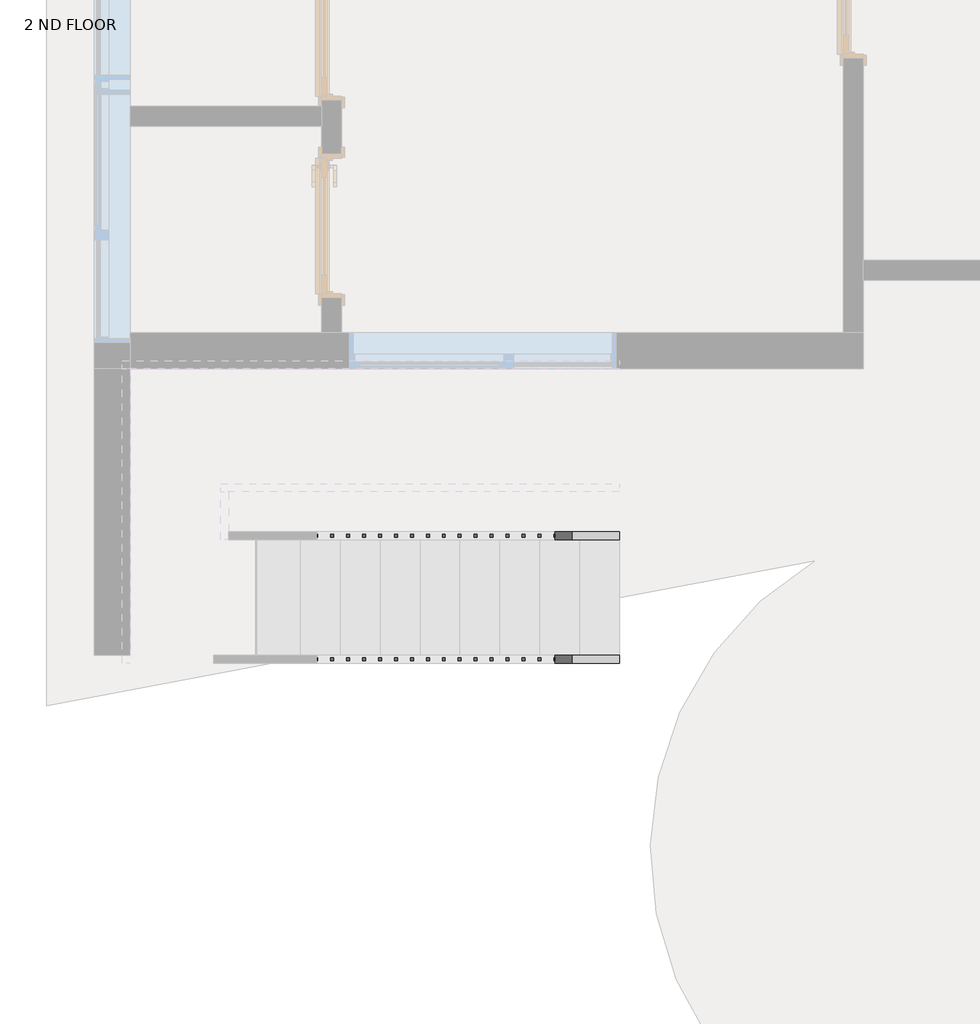
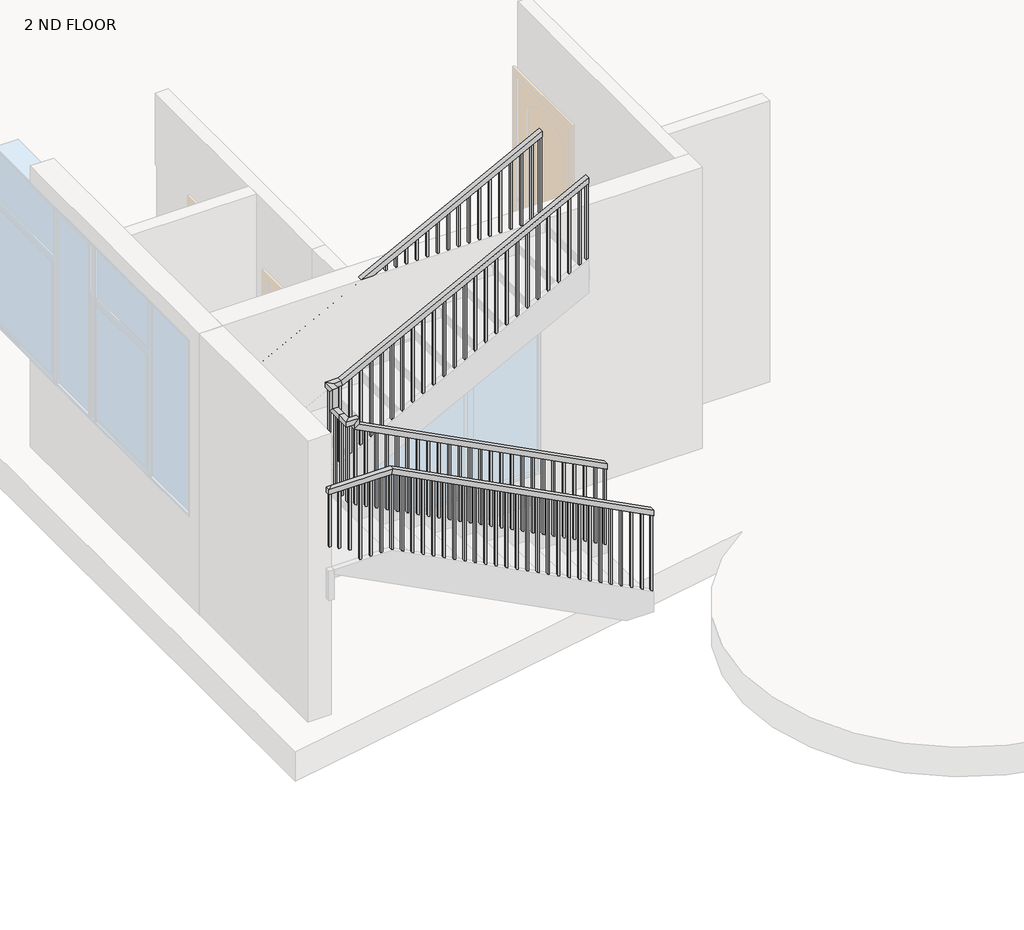
# One storey, part 3 of 4: 2 railings.
"""IFC4 building model written with IfcOpenShell, lengths in millimetres."""

from ifc_helpers import new_model, si_unit, frame, origin, place, context, project, spatial, polyline, outline, extrude, faceted_brep, element, save

model = new_model("IFC4")

# Units and contexts
model_context = context("Model", 3, world=origin())
ifc_project = project(units=[si_unit("LENGTHUNIT", "METRE", prefix="MILLI")], contexts=[model_context])

# Site, building, storey
site = spatial("IfcSite", under=ifc_project)
building = spatial("IfcBuilding", under=site)
storey = spatial("IfcBuildingStorey", under=building, Name="2 ND FLOOR", Elevation=6400.8)

# Railings
placement = place(None, origin())
element("IfcRailing", 1, ObjectType="Handrail - Rectangular", at=placement, inside=storey, context=model_context, shape_type="SolidModel", body=[
    faceted_brep([(-3117.2664982, -6914.3822004, 7446.8181818), (-3117.2664982, -6914.3822004, 7389.603028), (-3117.2664982, -6863.5822004, 7389.603028), (-3117.2664982, -6863.5822004, 7446.8181818), (-5530.2664982, -6914.3822004, 8697.1909091), (-5581.0664982, -6914.3822004, 8666.2993916), (-5581.0664982, -6863.5822004, 8666.2993916), (-5530.2664982, -6863.5822004, 8697.1909091), (-5657.2664982, -6787.3822004, 8712.2), (-5657.2664982, -6787.3822004, 8763.0), (-5657.2664982, -6685.7822004, 8763.0), (-5657.2664982, -6634.9822004, 8712.2), (-5606.4664982, -6787.3822004, 8712.2), (-5606.4664982, -6634.9822004, 8712.2), (-5606.4664982, -6787.3822004, 8763.0), (-5606.4664982, -6685.7822004, 8763.0), (-3117.2664982, -6558.7822004, 10210.8), (-3117.2664982, -6609.5822004, 10210.8), (-3117.2664982, -6609.5822004, 10153.5848461), (-3117.2664982, -6558.7822004, 10153.5848461), (-5517.8863767, -6558.7822004, 8909.6272727), (-5530.2664982, -6558.7822004, 8960.4272727), (-5517.8863767, -6609.5822004, 8909.6272727), (-5530.2664982, -6609.5822004, 8960.4272727), (-5530.2664982, -6914.3822004, 8763.0), (-5581.0664982, -6914.3822004, 8712.2), (-5581.0664982, -6863.5822004, 8712.2), (-5530.2664982, -6863.5822004, 8763.0), (-5657.2664982, -6914.3822004, 8763.0), (-5657.2664982, -6914.3822004, 8712.2), (-5606.4664982, -6863.5822004, 8712.2), (-5606.4664982, -6863.5822004, 8763.0), (-5657.2664982, -6685.7822004, 8960.4272727), (-5657.2664982, -6634.9822004, 8909.6272727), (-5606.4664982, -6634.9822004, 8909.6272727), (-5606.4664982, -6685.7822004, 8960.4272727), (-5657.2664982, -6558.7822004, 8960.4272727), (-5657.2664982, -6558.7822004, 8909.6272727), (-5606.4664982, -6609.5822004, 8909.6272727), (-5606.4664982, -6609.5822004, 8960.4272727)], [[[0, 1, 2, 3]], [[1, 0, 4, 5]], [[2, 1, 5, 6]], [[3, 2, 6, 7]], [[0, 3, 7, 4]], [[8, 9, 10, 11]], [[12, 8, 11, 13]], [[14, 12, 13, 15]], [[9, 14, 15, 10]], [[16, 17, 18, 19]], [[20, 21, 16, 19]], [[22, 20, 19, 18]], [[23, 22, 18, 17]], [[21, 23, 17, 16]], [[5, 4, 24, 25]], [[6, 5, 25, 26]], [[7, 6, 26, 27]], [[4, 7, 27, 24]], [[25, 24, 28, 29]], [[26, 25, 29, 30]], [[27, 26, 30, 31]], [[24, 27, 31, 28]], [[29, 28, 9, 8]], [[30, 29, 8, 12]], [[31, 30, 12, 14]], [[28, 31, 14, 9]], [[11, 10, 32, 33]], [[13, 11, 33, 34]], [[15, 13, 34, 35]], [[10, 15, 35, 32]], [[33, 32, 36, 37]], [[34, 33, 37, 38]], [[35, 34, 38, 39]], [[32, 35, 39, 36]], [[37, 36, 21, 20]], [[38, 37, 20, 22]], [[39, 38, 22, 23]], [[36, 39, 23, 21]]]),
    extrude(outline(polyline([(10119.0350734, -3183.9414982), (10109.1637098, -3202.9914982), (9324.8803899, -3202.9914982), (9334.7517536, -3183.9414982), (10119.0350734, -3183.9414982)])), frame((0.0, -6593.7072004, 0.0), z_axis=(0.0, 1.0, 0.0), x_axis=(0.0, 0.0, 1.0)), (0.0, 0.0, 1.0), 19.05),
    extrude(outline(polyline([(10066.3878007, -3285.5414982), (10056.516437, -3304.5914982), (9272.2331172, -3304.5914982), (9282.1044808, -3285.5414982), (10066.3878007, -3285.5414982)])), frame((0.0, -6593.7072004, 0.0), z_axis=(0.0, 1.0, 0.0), x_axis=(0.0, 0.0, 1.0)), (0.0, 0.0, 1.0), 19.05),
    extrude(outline(polyline([(10013.740528, -3387.1414982), (10003.8691643, -3406.1914982), (9219.5858445, -3406.1914982), (9229.4572081, -3387.1414982), (10013.740528, -3387.1414982)])), frame((0.0, -6593.7072004, 0.0), z_axis=(0.0, 1.0, 0.0), x_axis=(0.0, 0.0, 1.0)), (0.0, 0.0, 1.0), 19.05),
    extrude(outline(polyline([(9961.0932552, -3488.7414982), (9951.2218916, -3507.7914982), (9166.9385718, -3507.7914982), (9176.8099354, -3488.7414982), (9961.0932552, -3488.7414982)])), frame((0.0, -6593.7072004, 0.0), z_axis=(0.0, 1.0, 0.0), x_axis=(0.0, 0.0, 1.0)), (0.0, 0.0, 1.0), 19.05),
    extrude(outline(polyline([(9908.4459825, -3590.3414982), (9898.5746189, -3609.3914982), (9114.291299, -3609.3914982), (9124.1626627, -3590.3414982), (9908.4459825, -3590.3414982)])), frame((0.0, -6593.7072004, 0.0), z_axis=(0.0, 1.0, 0.0), x_axis=(0.0, 0.0, 1.0)), (0.0, 0.0, 1.0), 19.05),
    extrude(outline(polyline([(9855.7987098, -3691.9414982), (9845.9273461, -3710.9914982), (9061.6440263, -3710.9914982), (9071.5153899, -3691.9414982), (9855.7987098, -3691.9414982)])), frame((0.0, -6593.7072004, 0.0), z_axis=(0.0, 1.0, 0.0), x_axis=(0.0, 0.0, 1.0)), (0.0, 0.0, 1.0), 19.05),
    extrude(outline(polyline([(9803.151437, -3793.5414982), (9793.2800734, -3812.5914982), (9008.9967536, -3812.5914982), (9018.8681172, -3793.5414982), (9803.151437, -3793.5414982)])), frame((0.0, -6593.7072004, 0.0), z_axis=(0.0, 1.0, 0.0), x_axis=(0.0, 0.0, 1.0)), (0.0, 0.0, 1.0), 19.05),
    extrude(outline(polyline([(9750.5041643, -3895.1414982), (9740.6328007, -3914.1914982), (8956.3494808, -3914.1914982), (8966.2208445, -3895.1414982), (9750.5041643, -3895.1414982)])), frame((0.0, -6593.7072004, 0.0), z_axis=(0.0, 1.0, 0.0), x_axis=(0.0, 0.0, 1.0)), (0.0, 0.0, 1.0), 19.05),
    extrude(outline(polyline([(9697.8568916, -3996.7414982), (9687.985528, -4015.7914982), (8903.7022081, -4015.7914982), (8913.5735718, -3996.7414982), (9697.8568916, -3996.7414982)])), frame((0.0, -6593.7072004, 0.0), z_axis=(0.0, 1.0, 0.0), x_axis=(0.0, 0.0, 1.0)), (0.0, 0.0, 1.0), 19.05),
    extrude(outline(polyline([(9645.2096189, -4098.3414982), (9635.3382552, -4117.3914982), (8851.0549354, -4117.3914982), (8860.926299, -4098.3414982), (9645.2096189, -4098.3414982)])), frame((0.0, -6593.7072004, 0.0), z_axis=(0.0, 1.0, 0.0), x_axis=(0.0, 0.0, 1.0)), (0.0, 0.0, 1.0), 19.05),
    extrude(outline(polyline([(9592.5623461, -4199.9414982), (9582.6909825, -4218.9914982), (8798.4076627, -4218.9914982), (8808.2790263, -4199.9414982), (9592.5623461, -4199.9414982)])), frame((0.0, -6593.7072004, 0.0), z_axis=(0.0, 1.0, 0.0), x_axis=(0.0, 0.0, 1.0)), (0.0, 0.0, 1.0), 19.05),
    extrude(outline(polyline([(9539.9150734, -4301.5414982), (9530.0437098, -4320.5914982), (8745.7603899, -4320.5914982), (8755.6317536, -4301.5414982), (9539.9150734, -4301.5414982)])), frame((0.0, -6593.7072004, 0.0), z_axis=(0.0, 1.0, 0.0), x_axis=(0.0, 0.0, 1.0)), (0.0, 0.0, 1.0), 19.05),
    extrude(outline(polyline([(9487.2678007, -4403.1414982), (9477.396437, -4422.1914982), (8693.1131172, -4422.1914982), (8702.9844808, -4403.1414982), (9487.2678007, -4403.1414982)])), frame((0.0, -6593.7072004, 0.0), z_axis=(0.0, 1.0, 0.0), x_axis=(0.0, 0.0, 1.0)), (0.0, 0.0, 1.0), 19.05),
    extrude(outline(polyline([(9434.620528, -4504.7414982), (9424.7491643, -4523.7914982), (8640.4658445, -4523.7914982), (8650.3372081, -4504.7414982), (9434.620528, -4504.7414982)])), frame((0.0, -6593.7072004, 0.0), z_axis=(0.0, 1.0, 0.0), x_axis=(0.0, 0.0, 1.0)), (0.0, 0.0, 1.0), 19.05),
    extrude(outline(polyline([(9381.9732552, -4606.3414982), (9372.1018916, -4625.3914982), (8587.8185718, -4625.3914982), (8597.6899354, -4606.3414982), (9381.9732552, -4606.3414982)])), frame((0.0, -6593.7072004, 0.0), z_axis=(0.0, 1.0, 0.0), x_axis=(0.0, 0.0, 1.0)), (0.0, 0.0, 1.0), 19.05),
    extrude(outline(polyline([(9329.3259825, -4707.9414982), (9319.4546189, -4726.9914982), (8535.171299, -4726.9914982), (8545.0426627, -4707.9414982), (9329.3259825, -4707.9414982)])), frame((0.0, -6593.7072004, 0.0), z_axis=(0.0, 1.0, 0.0), x_axis=(0.0, 0.0, 1.0)), (0.0, 0.0, 1.0), 19.05),
    extrude(outline(polyline([(9276.6787098, -4809.5414982), (9266.8073461, -4828.5914982), (8482.5240263, -4828.5914982), (8492.3953899, -4809.5414982), (9276.6787098, -4809.5414982)])), frame((0.0, -6593.7072004, 0.0), z_axis=(0.0, 1.0, 0.0), x_axis=(0.0, 0.0, 1.0)), (0.0, 0.0, 1.0), 19.05),
    extrude(outline(polyline([(9224.031437, -4911.1414982), (9214.1600734, -4930.1914982), (8429.8767536, -4930.1914982), (8439.7481172, -4911.1414982), (9224.031437, -4911.1414982)])), frame((0.0, -6593.7072004, 0.0), z_axis=(0.0, 1.0, 0.0), x_axis=(0.0, 0.0, 1.0)), (0.0, 0.0, 1.0), 19.05),
    extrude(outline(polyline([(9171.3841643, -5012.7414982), (9161.5128007, -5031.7914982), (8377.2294808, -5031.7914982), (8387.1008445, -5012.7414982), (9171.3841643, -5012.7414982)])), frame((0.0, -6593.7072004, 0.0), z_axis=(0.0, 1.0, 0.0), x_axis=(0.0, 0.0, 1.0)), (0.0, 0.0, 1.0), 19.05),
    extrude(outline(polyline([(9118.7368916, -5114.3414982), (9108.865528, -5133.3914982), (8324.5822081, -5133.3914982), (8334.4535718, -5114.3414982), (9118.7368916, -5114.3414982)])), frame((0.0, -6593.7072004, 0.0), z_axis=(0.0, 1.0, 0.0), x_axis=(0.0, 0.0, 1.0)), (0.0, 0.0, 1.0), 19.05),
    extrude(outline(polyline([(9066.0896189, -5215.9414982), (9056.2182552, -5234.9914982), (8271.9349354, -5234.9914982), (8281.806299, -5215.9414982), (9066.0896189, -5215.9414982)])), frame((0.0, -6593.7072004, 0.0), z_axis=(0.0, 1.0, 0.0), x_axis=(0.0, 0.0, 1.0)), (0.0, 0.0, 1.0), 19.05),
    extrude(outline(polyline([(9013.4423461, -5317.5414982), (9003.5709825, -5336.5914982), (8219.2876627, -5336.5914982), (8229.1590263, -5317.5414982), (9013.4423461, -5317.5414982)])), frame((0.0, -6593.7072004, 0.0), z_axis=(0.0, 1.0, 0.0), x_axis=(0.0, 0.0, 1.0)), (0.0, 0.0, 1.0), 19.05),
    extrude(outline(polyline([(8960.7950734, -5419.1414982), (8950.9237098, -5438.1914982), (8166.6403899, -5438.1914982), (8176.5117536, -5419.1414982), (8960.7950734, -5419.1414982)])), frame((0.0, -6593.7072004, 0.0), z_axis=(0.0, 1.0, 0.0), x_axis=(0.0, 0.0, 1.0)), (0.0, 0.0, 1.0), 19.05),
    extrude(outline(polyline([(8908.1478007, -5520.7414982), (8898.276437, -5539.7914982), (8113.9931172, -5539.7914982), (8123.8644808, -5520.7414982), (8908.1478007, -5520.7414982)])), frame((0.0, -6593.7072004, 0.0), z_axis=(0.0, 1.0, 0.0), x_axis=(0.0, 0.0, 1.0)), (0.0, 0.0, 1.0), 19.05),
    extrude(outline(polyline([(-5622.3414982, -6695.3072004), (-5641.3914982, -6695.3072004), (-5641.3914982, -6676.2572004), (-5622.3414982, -6676.2572004), (-5622.3414982, -6695.3072004)])), frame((0.0, 0.0, 7924.8), z_axis=(0.0, 0.0, 1.0), x_axis=(1.0, 0.0, 0.0)), (0.0, 0.0, 1.0), 787.4),
    extrude(outline(polyline([(-5622.3414982, -6796.9072004), (-5641.3914982, -6796.9072004), (-5641.3914982, -6777.8572004), (-5622.3414982, -6777.8572004), (-5622.3414982, -6796.9072004)])), frame((0.0, 0.0, 7924.8), z_axis=(0.0, 0.0, 1.0), x_axis=(1.0, 0.0, 0.0)), (0.0, 0.0, 1.0), 787.4),
    extrude(outline(polyline([(8712.2, -5546.1414982), (8712.2, -5565.1914982), (7873.7899354, -5565.1914982), (7863.9185718, -5546.1414982), (8712.2, -5546.1414982)])), frame((0.0, -6898.5072004, 0.0), z_axis=(0.0, 1.0, 0.0), x_axis=(0.0, 0.0, 1.0)), (0.0, 0.0, 1.0), 19.05),
    extrude(outline(polyline([(8595.5546189, -5444.5414982), (8605.4259825, -5463.5914982), (7821.1426627, -5463.5914982), (7811.271299, -5444.5414982), (8595.5546189, -5444.5414982)])), frame((0.0, -6898.5072004, 0.0), z_axis=(0.0, 1.0, 0.0), x_axis=(0.0, 0.0, 1.0)), (0.0, 0.0, 1.0), 19.05),
    extrude(outline(polyline([(8542.9073461, -5342.9414982), (8552.7787098, -5361.9914982), (7768.4953899, -5361.9914982), (7758.6240263, -5342.9414982), (8542.9073461, -5342.9414982)])), frame((0.0, -6898.5072004, 0.0), z_axis=(0.0, 1.0, 0.0), x_axis=(0.0, 0.0, 1.0)), (0.0, 0.0, 1.0), 19.05),
    extrude(outline(polyline([(8490.2600734, -5241.3414982), (8500.131437, -5260.3914982), (7715.8481172, -5260.3914982), (7705.9767536, -5241.3414982), (8490.2600734, -5241.3414982)])), frame((0.0, -6898.5072004, 0.0), z_axis=(0.0, 1.0, 0.0), x_axis=(0.0, 0.0, 1.0)), (0.0, 0.0, 1.0), 19.05),
    extrude(outline(polyline([(8437.6128007, -5139.7414982), (8447.4841643, -5158.7914982), (7663.2008445, -5158.7914982), (7653.3294808, -5139.7414982), (8437.6128007, -5139.7414982)])), frame((0.0, -6898.5072004, 0.0), z_axis=(0.0, 1.0, 0.0), x_axis=(0.0, 0.0, 1.0)), (0.0, 0.0, 1.0), 19.05),
    extrude(outline(polyline([(8384.965528, -5038.1414982), (8394.8368916, -5057.1914982), (7610.5535718, -5057.1914982), (7600.6822081, -5038.1414982), (8384.965528, -5038.1414982)])), frame((0.0, -6898.5072004, 0.0), z_axis=(0.0, 1.0, 0.0), x_axis=(0.0, 0.0, 1.0)), (0.0, 0.0, 1.0), 19.05),
    extrude(outline(polyline([(8332.3182552, -4936.5414982), (8342.1896189, -4955.5914982), (7557.906299, -4955.5914982), (7548.0349354, -4936.5414982), (8332.3182552, -4936.5414982)])), frame((0.0, -6898.5072004, 0.0), z_axis=(0.0, 1.0, 0.0), x_axis=(0.0, 0.0, 1.0)), (0.0, 0.0, 1.0), 19.05),
    extrude(outline(polyline([(8279.6709825, -4834.9414982), (8289.5423461, -4853.9914982), (7505.2590263, -4853.9914982), (7495.3876627, -4834.9414982), (8279.6709825, -4834.9414982)])), frame((0.0, -6898.5072004, 0.0), z_axis=(0.0, 1.0, 0.0), x_axis=(0.0, 0.0, 1.0)), (0.0, 0.0, 1.0), 19.05),
    extrude(outline(polyline([(8227.0237098, -4733.3414982), (8236.8950734, -4752.3914982), (7452.6117536, -4752.3914982), (7442.7403899, -4733.3414982), (8227.0237098, -4733.3414982)])), frame((0.0, -6898.5072004, 0.0), z_axis=(0.0, 1.0, 0.0), x_axis=(0.0, 0.0, 1.0)), (0.0, 0.0, 1.0), 19.05),
    extrude(outline(polyline([(8174.376437, -4631.7414982), (8184.2478007, -4650.7914982), (7399.9644808, -4650.7914982), (7390.0931172, -4631.7414982), (8174.376437, -4631.7414982)])), frame((0.0, -6898.5072004, 0.0), z_axis=(0.0, 1.0, 0.0), x_axis=(0.0, 0.0, 1.0)), (0.0, 0.0, 1.0), 19.05),
    extrude(outline(polyline([(8121.7291643, -4530.1414982), (8131.600528, -4549.1914982), (7347.3172081, -4549.1914982), (7337.4458445, -4530.1414982), (8121.7291643, -4530.1414982)])), frame((0.0, -6898.5072004, 0.0), z_axis=(0.0, 1.0, 0.0), x_axis=(0.0, 0.0, 1.0)), (0.0, 0.0, 1.0), 19.05),
    extrude(outline(polyline([(8069.0818916, -4428.5414982), (8078.9532552, -4447.5914982), (7294.6699354, -4447.5914982), (7284.7985718, -4428.5414982), (8069.0818916, -4428.5414982)])), frame((0.0, -6898.5072004, 0.0), z_axis=(0.0, 1.0, 0.0), x_axis=(0.0, 0.0, 1.0)), (0.0, 0.0, 1.0), 19.05),
    extrude(outline(polyline([(8016.4346189, -4326.9414982), (8026.3059825, -4345.9914982), (7242.0226627, -4345.9914982), (7232.151299, -4326.9414982), (8016.4346189, -4326.9414982)])), frame((0.0, -6898.5072004, 0.0), z_axis=(0.0, 1.0, 0.0), x_axis=(0.0, 0.0, 1.0)), (0.0, 0.0, 1.0), 19.05),
    extrude(outline(polyline([(7963.7873461, -4225.3414982), (7973.6587098, -4244.3914982), (7189.3753899, -4244.3914982), (7179.5040263, -4225.3414982), (7963.7873461, -4225.3414982)])), frame((0.0, -6898.5072004, 0.0), z_axis=(0.0, 1.0, 0.0), x_axis=(0.0, 0.0, 1.0)), (0.0, 0.0, 1.0), 19.05),
    extrude(outline(polyline([(7911.1400734, -4123.7414982), (7921.011437, -4142.7914982), (7136.7281172, -4142.7914982), (7126.8567536, -4123.7414982), (7911.1400734, -4123.7414982)])), frame((0.0, -6898.5072004, 0.0), z_axis=(0.0, 1.0, 0.0), x_axis=(0.0, 0.0, 1.0)), (0.0, 0.0, 1.0), 19.05),
    extrude(outline(polyline([(7858.4928007, -4022.1414982), (7868.3641643, -4041.1914982), (7084.0808445, -4041.1914982), (7074.2094808, -4022.1414982), (7858.4928007, -4022.1414982)])), frame((0.0, -6898.5072004, 0.0), z_axis=(0.0, 1.0, 0.0), x_axis=(0.0, 0.0, 1.0)), (0.0, 0.0, 1.0), 19.05),
    extrude(outline(polyline([(7805.845528, -3920.5414982), (7815.7168916, -3939.5914982), (7031.4335718, -3939.5914982), (7021.5622081, -3920.5414982), (7805.845528, -3920.5414982)])), frame((0.0, -6898.5072004, 0.0), z_axis=(0.0, 1.0, 0.0), x_axis=(0.0, 0.0, 1.0)), (0.0, 0.0, 1.0), 19.05),
    extrude(outline(polyline([(7753.1982552, -3818.9414982), (7763.0696189, -3837.9914982), (6978.786299, -3837.9914982), (6968.9149354, -3818.9414982), (7753.1982552, -3818.9414982)])), frame((0.0, -6898.5072004, 0.0), z_axis=(0.0, 1.0, 0.0), x_axis=(0.0, 0.0, 1.0)), (0.0, 0.0, 1.0), 19.05),
    extrude(outline(polyline([(7700.5509825, -3717.3414982), (7710.4223461, -3736.3914982), (6926.1390263, -3736.3914982), (6916.2676627, -3717.3414982), (7700.5509825, -3717.3414982)])), frame((0.0, -6898.5072004, 0.0), z_axis=(0.0, 1.0, 0.0), x_axis=(0.0, 0.0, 1.0)), (0.0, 0.0, 1.0), 19.05),
    extrude(outline(polyline([(7647.9037098, -3615.7414982), (7657.7750734, -3634.7914982), (6873.4917536, -3634.7914982), (6863.6203899, -3615.7414982), (7647.9037098, -3615.7414982)])), frame((0.0, -6898.5072004, 0.0), z_axis=(0.0, 1.0, 0.0), x_axis=(0.0, 0.0, 1.0)), (0.0, 0.0, 1.0), 19.05),
    extrude(outline(polyline([(7595.256437, -3514.1414982), (7605.1278007, -3533.1914982), (6820.8444808, -3533.1914982), (6810.9731172, -3514.1414982), (7595.256437, -3514.1414982)])), frame((0.0, -6898.5072004, 0.0), z_axis=(0.0, 1.0, 0.0), x_axis=(0.0, 0.0, 1.0)), (0.0, 0.0, 1.0), 19.05),
    extrude(outline(polyline([(7542.6091643, -3412.5414982), (7552.480528, -3431.5914982), (6768.1972081, -3431.5914982), (6758.3258445, -3412.5414982), (7542.6091643, -3412.5414982)])), frame((0.0, -6898.5072004, 0.0), z_axis=(0.0, 1.0, 0.0), x_axis=(0.0, 0.0, 1.0)), (0.0, 0.0, 1.0), 19.05),
    extrude(outline(polyline([(7489.9618916, -3310.9414982), (7499.8332552, -3329.9914982), (6715.5499354, -3329.9914982), (6705.6785718, -3310.9414982), (7489.9618916, -3310.9414982)])), frame((0.0, -6898.5072004, 0.0), z_axis=(0.0, 1.0, 0.0), x_axis=(0.0, 0.0, 1.0)), (0.0, 0.0, 1.0), 19.05),
    extrude(outline(polyline([(7437.3146189, -3209.3414982), (7447.1859825, -3228.3914982), (6662.9026627, -3228.3914982), (6653.031299, -3209.3414982), (7437.3146189, -3209.3414982)])), frame((0.0, -6898.5072004, 0.0), z_axis=(0.0, 1.0, 0.0), x_axis=(0.0, 0.0, 1.0)), (0.0, 0.0, 1.0), 19.05),
    extrude(outline(polyline([(-6593.7072004, 8909.6272727), (-6574.6572004, 8909.6272727), (-6574.6572004, 8071.2172081), (-6593.7072004, 8061.3458445), (-6593.7072004, 8909.6272727)])), frame((-5641.3914982, 0.0, 0.0), z_axis=(1.0, 0.0, 0.0), x_axis=(0.0, 1.0, 0.0)), (0.0, 0.0, 1.0), 19.05),
    extrude(outline(polyline([(-5622.3414982, -6879.4572004), (-5622.3414982, -6898.5072004), (-5641.3914982, -6898.5072004), (-5641.3914982, -6879.4572004), (-5622.3414982, -6879.4572004)])), frame((0.0, 0.0, 7924.8), z_axis=(0.0, 0.0, 1.0), x_axis=(1.0, 0.0, 0.0)), (0.0, 0.0, 1.0), 787.4),
    extrude(outline(polyline([(10153.5848461, -3117.2664982), (10143.7134825, -3136.3164982), (9359.4301627, -3136.3164982), (9369.3015263, -3117.2664982), (10153.5848461, -3117.2664982)])), frame((0.0, -6593.7072004, 0.0), z_axis=(0.0, 1.0, 0.0), x_axis=(0.0, 0.0, 1.0)), (0.0, 0.0, 1.0), 19.05),
    extrude(outline(polyline([(7389.603028, -3117.2664982), (7399.4743916, -3136.3164982), (6615.1910718, -3136.3164982), (6605.3197081, -3117.2664982), (7389.603028, -3117.2664982)])), frame((0.0, -6898.5072004, 0.0), z_axis=(0.0, 1.0, 0.0), x_axis=(0.0, 0.0, 1.0)), (0.0, 0.0, 1.0), 19.05),
])
element("IfcRailing", 2, ObjectType="Handrail - Rectangular", at=placement, inside=storey, context=model_context, shape_type="SolidModel", body=[
    faceted_brep([(-3117.2664982, -7701.7822004, 7446.8181818), (-3117.2664982, -7701.7822004, 7389.603028), (-3117.2664982, -7650.9822004, 7389.603028), (-3117.2664982, -7650.9822004, 7446.8181818), (-5657.2664982, -7701.7822004, 8763.0), (-5669.6466197, -7701.7822004, 8712.2), (-5669.6466197, -7650.9822004, 8712.2), (-5657.2664982, -7650.9822004, 8763.0), (-6283.3131972, -7701.7822004, 8712.2), (-6283.3131972, -7701.7822004, 8763.0), (-6283.3131972, -5773.9082131, 8763.0), (-6283.3131972, -5773.9082131, 8712.2), (-6232.5131972, -7650.9822004, 8712.2), (-6232.5131972, -5824.7082131, 8712.2), (-6232.5131972, -7650.9822004, 8763.0), (-6232.5131972, -5824.7082131, 8763.0), (-5911.2664982, -5773.9082131, 8763.0), (-5898.8863767, -5773.9082131, 8712.2), (-5898.8863767, -5824.7082131, 8712.2), (-5911.2664982, -5824.7082131, 8763.0), (-3117.2664982, -5773.9082131, 10210.8), (-3117.2664982, -5824.7082131, 10210.8), (-3117.2664982, -5824.7082131, 10153.5848461), (-3117.2664982, -5773.9082131, 10153.5848461)], [[[0, 1, 2, 3]], [[1, 0, 4, 5]], [[2, 1, 5, 6]], [[3, 2, 6, 7]], [[0, 3, 7, 4]], [[8, 9, 10, 11]], [[12, 8, 11, 13]], [[14, 12, 13, 15]], [[9, 14, 15, 10]], [[11, 10, 16, 17]], [[13, 11, 17, 18]], [[15, 13, 18, 19]], [[10, 15, 19, 16]], [[5, 4, 9, 8]], [[6, 5, 8, 12]], [[7, 6, 12, 14]], [[4, 7, 14, 9]], [[20, 21, 22, 23]], [[17, 16, 20, 23]], [[18, 17, 23, 22]], [[19, 18, 22, 21]], [[16, 19, 21, 20]]]),
    extrude(outline(polyline([(10100.6413294, -3219.4381972), (9316.3580095, -3219.4381972), (9326.2293732, -3200.3881972), (10110.512693, -3200.3881972), (10100.6413294, -3219.4381972)])), frame((0.0, -5808.8332131, 0.0), z_axis=(0.0, 1.0, 0.0), x_axis=(0.0, 0.0, 1.0)), (0.0, 0.0, 1.0), 19.05),
    extrude(outline(polyline([(10047.9940566, -3321.0381972), (9263.7107368, -3321.0381972), (9273.5821004, -3301.9881972), (10057.8654203, -3301.9881972), (10047.9940566, -3321.0381972)])), frame((0.0, -5808.8332131, 0.0), z_axis=(0.0, 1.0, 0.0), x_axis=(0.0, 0.0, 1.0)), (0.0, 0.0, 1.0), 19.05),
    extrude(outline(polyline([(9995.3467839, -3422.6381972), (9211.0634641, -3422.6381972), (9220.9348277, -3403.5881972), (10005.2181476, -3403.5881972), (9995.3467839, -3422.6381972)])), frame((0.0, -5808.8332131, 0.0), z_axis=(0.0, 1.0, 0.0), x_axis=(0.0, 0.0, 1.0)), (0.0, 0.0, 1.0), 19.05),
    extrude(outline(polyline([(9942.6995112, -3524.2381972), (9158.4161913, -3524.2381972), (9168.287555, -3505.1881972), (9952.5708748, -3505.1881972), (9942.6995112, -3524.2381972)])), frame((0.0, -5808.8332131, 0.0), z_axis=(0.0, 1.0, 0.0), x_axis=(0.0, 0.0, 1.0)), (0.0, 0.0, 1.0), 19.05),
    extrude(outline(polyline([(9890.0522385, -3625.8381972), (9105.7689186, -3625.8381972), (9115.6402823, -3606.7881972), (9899.9236021, -3606.7881972), (9890.0522385, -3625.8381972)])), frame((0.0, -5808.8332131, 0.0), z_axis=(0.0, 1.0, 0.0), x_axis=(0.0, 0.0, 1.0)), (0.0, 0.0, 1.0), 19.05),
    extrude(outline(polyline([(9837.4049657, -3727.4381972), (9053.1216459, -3727.4381972), (9062.9930095, -3708.3881972), (9847.2763294, -3708.3881972), (9837.4049657, -3727.4381972)])), frame((0.0, -5808.8332131, 0.0), z_axis=(0.0, 1.0, 0.0), x_axis=(0.0, 0.0, 1.0)), (0.0, 0.0, 1.0), 19.05),
    extrude(outline(polyline([(9784.757693, -3829.0381972), (9000.4743732, -3829.0381972), (9010.3457368, -3809.9881972), (9794.6290566, -3809.9881972), (9784.757693, -3829.0381972)])), frame((0.0, -5808.8332131, 0.0), z_axis=(0.0, 1.0, 0.0), x_axis=(0.0, 0.0, 1.0)), (0.0, 0.0, 1.0), 19.05),
    extrude(outline(polyline([(9732.1104203, -3930.6381972), (8947.8271004, -3930.6381972), (8957.6984641, -3911.5881972), (9741.9817839, -3911.5881972), (9732.1104203, -3930.6381972)])), frame((0.0, -5808.8332131, 0.0), z_axis=(0.0, 1.0, 0.0), x_axis=(0.0, 0.0, 1.0)), (0.0, 0.0, 1.0), 19.05),
    extrude(outline(polyline([(9679.4631476, -4032.2381972), (8895.1798277, -4032.2381972), (8905.0511913, -4013.1881972), (9689.3345112, -4013.1881972), (9679.4631476, -4032.2381972)])), frame((0.0, -5808.8332131, 0.0), z_axis=(0.0, 1.0, 0.0), x_axis=(0.0, 0.0, 1.0)), (0.0, 0.0, 1.0), 19.05),
    extrude(outline(polyline([(9626.8158748, -4133.8381972), (8842.532555, -4133.8381972), (8852.4039186, -4114.7881972), (9636.6872385, -4114.7881972), (9626.8158748, -4133.8381972)])), frame((0.0, -5808.8332131, 0.0), z_axis=(0.0, 1.0, 0.0), x_axis=(0.0, 0.0, 1.0)), (0.0, 0.0, 1.0), 19.05),
    extrude(outline(polyline([(9574.1686021, -4235.4381972), (8789.8852823, -4235.4381972), (8799.7566459, -4216.3881972), (9584.0399657, -4216.3881972), (9574.1686021, -4235.4381972)])), frame((0.0, -5808.8332131, 0.0), z_axis=(0.0, 1.0, 0.0), x_axis=(0.0, 0.0, 1.0)), (0.0, 0.0, 1.0), 19.05),
    extrude(outline(polyline([(9521.5213294, -4337.0381972), (8737.2380095, -4337.0381972), (8747.1093732, -4317.9881972), (9531.392693, -4317.9881972), (9521.5213294, -4337.0381972)])), frame((0.0, -5808.8332131, 0.0), z_axis=(0.0, 1.0, 0.0), x_axis=(0.0, 0.0, 1.0)), (0.0, 0.0, 1.0), 19.05),
    extrude(outline(polyline([(9468.8740566, -4438.6381972), (8684.5907368, -4438.6381972), (8694.4621004, -4419.5881972), (9478.7454203, -4419.5881972), (9468.8740566, -4438.6381972)])), frame((0.0, -5808.8332131, 0.0), z_axis=(0.0, 1.0, 0.0), x_axis=(0.0, 0.0, 1.0)), (0.0, 0.0, 1.0), 19.05),
    extrude(outline(polyline([(9416.2267839, -4540.2381972), (8631.9434641, -4540.2381972), (8641.8148277, -4521.1881972), (9426.0981476, -4521.1881972), (9416.2267839, -4540.2381972)])), frame((0.0, -5808.8332131, 0.0), z_axis=(0.0, 1.0, 0.0), x_axis=(0.0, 0.0, 1.0)), (0.0, 0.0, 1.0), 19.05),
    extrude(outline(polyline([(9363.5795112, -4641.8381972), (8579.2961913, -4641.8381972), (8589.167555, -4622.7881972), (9373.4508748, -4622.7881972), (9363.5795112, -4641.8381972)])), frame((0.0, -5808.8332131, 0.0), z_axis=(0.0, 1.0, 0.0), x_axis=(0.0, 0.0, 1.0)), (0.0, 0.0, 1.0), 19.05),
    extrude(outline(polyline([(9310.9322385, -4743.4381972), (8526.6489186, -4743.4381972), (8536.5202823, -4724.3881972), (9320.8036021, -4724.3881972), (9310.9322385, -4743.4381972)])), frame((0.0, -5808.8332131, 0.0), z_axis=(0.0, 1.0, 0.0), x_axis=(0.0, 0.0, 1.0)), (0.0, 0.0, 1.0), 19.05),
    extrude(outline(polyline([(9258.2849657, -4845.0381972), (8474.0016459, -4845.0381972), (8483.8730095, -4825.9881972), (9268.1563294, -4825.9881972), (9258.2849657, -4845.0381972)])), frame((0.0, -5808.8332131, 0.0), z_axis=(0.0, 1.0, 0.0), x_axis=(0.0, 0.0, 1.0)), (0.0, 0.0, 1.0), 19.05),
    extrude(outline(polyline([(9205.637693, -4946.6381972), (8421.3543732, -4946.6381972), (8431.2257368, -4927.5881972), (9215.5090566, -4927.5881972), (9205.637693, -4946.6381972)])), frame((0.0, -5808.8332131, 0.0), z_axis=(0.0, 1.0, 0.0), x_axis=(0.0, 0.0, 1.0)), (0.0, 0.0, 1.0), 19.05),
    extrude(outline(polyline([(9152.9904203, -5048.2381972), (8368.7071004, -5048.2381972), (8378.5784641, -5029.1881972), (9162.8617839, -5029.1881972), (9152.9904203, -5048.2381972)])), frame((0.0, -5808.8332131, 0.0), z_axis=(0.0, 1.0, 0.0), x_axis=(0.0, 0.0, 1.0)), (0.0, 0.0, 1.0), 19.05),
    extrude(outline(polyline([(9100.3431476, -5149.8381972), (8316.0598277, -5149.8381972), (8325.9311913, -5130.7881972), (9110.2145112, -5130.7881972), (9100.3431476, -5149.8381972)])), frame((0.0, -5808.8332131, 0.0), z_axis=(0.0, 1.0, 0.0), x_axis=(0.0, 0.0, 1.0)), (0.0, 0.0, 1.0), 19.05),
    extrude(outline(polyline([(9047.6958748, -5251.4381972), (8263.412555, -5251.4381972), (8273.2839186, -5232.3881972), (9057.5672385, -5232.3881972), (9047.6958748, -5251.4381972)])), frame((0.0, -5808.8332131, 0.0), z_axis=(0.0, 1.0, 0.0), x_axis=(0.0, 0.0, 1.0)), (0.0, 0.0, 1.0), 19.05),
    extrude(outline(polyline([(8995.0486021, -5353.0381972), (8210.7652823, -5353.0381972), (8220.6366459, -5333.9881972), (9004.9199657, -5333.9881972), (8995.0486021, -5353.0381972)])), frame((0.0, -5808.8332131, 0.0), z_axis=(0.0, 1.0, 0.0), x_axis=(0.0, 0.0, 1.0)), (0.0, 0.0, 1.0), 19.05),
    extrude(outline(polyline([(8942.4013294, -5454.6381972), (8158.1180095, -5454.6381972), (8167.9893732, -5435.5881972), (8952.272693, -5435.5881972), (8942.4013294, -5454.6381972)])), frame((0.0, -5808.8332131, 0.0), z_axis=(0.0, 1.0, 0.0), x_axis=(0.0, 0.0, 1.0)), (0.0, 0.0, 1.0), 19.05),
    extrude(outline(polyline([(8889.7540566, -5556.2381972), (8105.4707368, -5556.2381972), (8115.3421004, -5537.1881972), (8899.6254203, -5537.1881972), (8889.7540566, -5556.2381972)])), frame((0.0, -5808.8332131, 0.0), z_axis=(0.0, 1.0, 0.0), x_axis=(0.0, 0.0, 1.0)), (0.0, 0.0, 1.0), 19.05),
    extrude(outline(polyline([(8837.1067839, -5657.8381972), (8052.8234641, -5657.8381972), (8062.6948277, -5638.7881972), (8846.9781476, -5638.7881972), (8837.1067839, -5657.8381972)])), frame((0.0, -5808.8332131, 0.0), z_axis=(0.0, 1.0, 0.0), x_axis=(0.0, 0.0, 1.0)), (0.0, 0.0, 1.0), 19.05),
    extrude(outline(polyline([(8784.4595112, -5759.4381972), (8000.1761913, -5759.4381972), (8010.047555, -5740.3881972), (8794.3308748, -5740.3881972), (8784.4595112, -5759.4381972)])), frame((0.0, -5808.8332131, 0.0), z_axis=(0.0, 1.0, 0.0), x_axis=(0.0, 0.0, 1.0)), (0.0, 0.0, 1.0), 19.05),
    extrude(outline(polyline([(8731.8122385, -5861.0381972), (7947.5289186, -5861.0381972), (7957.4002823, -5841.9881972), (8741.6836021, -5841.9881972), (8731.8122385, -5861.0381972)])), frame((0.0, -5808.8332131, 0.0), z_axis=(0.0, 1.0, 0.0), x_axis=(0.0, 0.0, 1.0)), (0.0, 0.0, 1.0), 19.05),
    extrude(outline(polyline([(8712.2, -5962.6381972), (7894.8816459, -5962.6381972), (7904.7530095, -5943.5881972), (8712.2, -5943.5881972), (8712.2, -5962.6381972)])), frame((0.0, -5808.8332131, 0.0), z_axis=(0.0, 1.0, 0.0), x_axis=(0.0, 0.0, 1.0)), (0.0, 0.0, 1.0), 19.05),
    extrude(outline(polyline([(8712.2, -6064.2381972), (7842.2343732, -6064.2381972), (7852.1057368, -6045.1881972), (8712.2, -6045.1881972), (8712.2, -6064.2381972)])), frame((0.0, -5808.8332131, 0.0), z_axis=(0.0, 1.0, 0.0), x_axis=(0.0, 0.0, 1.0)), (0.0, 0.0, 1.0), 19.05),
    extrude(outline(polyline([(8712.2, -6165.8381972), (7789.5871004, -6165.8381972), (7799.4584641, -6146.7881972), (8712.2, -6146.7881972), (8712.2, -6165.8381972)])), frame((0.0, -5808.8332131, 0.0), z_axis=(0.0, 1.0, 0.0), x_axis=(0.0, 0.0, 1.0)), (0.0, 0.0, 1.0), 19.05),
    extrude(outline(polyline([(-6267.4381972, -5857.1072004), (-6267.4381972, -5838.0572004), (-6248.3881972, -5838.0572004), (-6248.3881972, -5857.1072004), (-6267.4381972, -5857.1072004)])), frame((0.0, 0.0, 7924.8), z_axis=(0.0, 0.0, 1.0), x_axis=(1.0, 0.0, 0.0)), (0.0, 0.0, 1.0), 787.4),
    extrude(outline(polyline([(-6267.4381972, -5958.7072004), (-6267.4381972, -5939.6572004), (-6248.3881972, -5939.6572004), (-6248.3881972, -5958.7072004), (-6267.4381972, -5958.7072004)])), frame((0.0, 0.0, 7924.8), z_axis=(0.0, 0.0, 1.0), x_axis=(1.0, 0.0, 0.0)), (0.0, 0.0, 1.0), 787.4),
    extrude(outline(polyline([(-6267.4381972, -6060.3072004), (-6267.4381972, -6041.2572004), (-6248.3881972, -6041.2572004), (-6248.3881972, -6060.3072004), (-6267.4381972, -6060.3072004)])), frame((0.0, 0.0, 7924.8), z_axis=(0.0, 0.0, 1.0), x_axis=(1.0, 0.0, 0.0)), (0.0, 0.0, 1.0), 787.4),
    extrude(outline(polyline([(-6267.4381972, -6161.9072004), (-6267.4381972, -6142.8572004), (-6248.3881972, -6142.8572004), (-6248.3881972, -6161.9072004), (-6267.4381972, -6161.9072004)])), frame((0.0, 0.0, 7924.8), z_axis=(0.0, 0.0, 1.0), x_axis=(1.0, 0.0, 0.0)), (0.0, 0.0, 1.0), 787.4),
    extrude(outline(polyline([(-6267.4381972, -6263.5072004), (-6267.4381972, -6244.4572004), (-6248.3881972, -6244.4572004), (-6248.3881972, -6263.5072004), (-6267.4381972, -6263.5072004)])), frame((0.0, 0.0, 7924.8), z_axis=(0.0, 0.0, 1.0), x_axis=(1.0, 0.0, 0.0)), (0.0, 0.0, 1.0), 787.4),
    extrude(outline(polyline([(-6267.4381972, -6365.1072004), (-6267.4381972, -6346.0572004), (-6248.3881972, -6346.0572004), (-6248.3881972, -6365.1072004), (-6267.4381972, -6365.1072004)])), frame((0.0, 0.0, 7924.8), z_axis=(0.0, 0.0, 1.0), x_axis=(1.0, 0.0, 0.0)), (0.0, 0.0, 1.0), 787.4),
    extrude(outline(polyline([(-6267.4381972, -6466.7072004), (-6267.4381972, -6447.6572004), (-6248.3881972, -6447.6572004), (-6248.3881972, -6466.7072004), (-6267.4381972, -6466.7072004)])), frame((0.0, 0.0, 7924.8), z_axis=(0.0, 0.0, 1.0), x_axis=(1.0, 0.0, 0.0)), (0.0, 0.0, 1.0), 787.4),
    extrude(outline(polyline([(-6267.4381972, -6568.3072004), (-6267.4381972, -6549.2572004), (-6248.3881972, -6549.2572004), (-6248.3881972, -6568.3072004), (-6267.4381972, -6568.3072004)])), frame((0.0, 0.0, 7924.8), z_axis=(0.0, 0.0, 1.0), x_axis=(1.0, 0.0, 0.0)), (0.0, 0.0, 1.0), 787.4),
    extrude(outline(polyline([(-6267.4381972, -6669.9072004), (-6267.4381972, -6650.8572004), (-6248.3881972, -6650.8572004), (-6248.3881972, -6669.9072004), (-6267.4381972, -6669.9072004)])), frame((0.0, 0.0, 7924.8), z_axis=(0.0, 0.0, 1.0), x_axis=(1.0, 0.0, 0.0)), (0.0, 0.0, 1.0), 787.4),
    extrude(outline(polyline([(-6267.4381972, -6771.5072004), (-6267.4381972, -6752.4572004), (-6248.3881972, -6752.4572004), (-6248.3881972, -6771.5072004), (-6267.4381972, -6771.5072004)])), frame((0.0, 0.0, 7924.8), z_axis=(0.0, 0.0, 1.0), x_axis=(1.0, 0.0, 0.0)), (0.0, 0.0, 1.0), 787.4),
    extrude(outline(polyline([(-6267.4381972, -6873.1072004), (-6267.4381972, -6854.0572004), (-6248.3881972, -6854.0572004), (-6248.3881972, -6873.1072004), (-6267.4381972, -6873.1072004)])), frame((0.0, 0.0, 7924.8), z_axis=(0.0, 0.0, 1.0), x_axis=(1.0, 0.0, 0.0)), (0.0, 0.0, 1.0), 787.4),
    extrude(outline(polyline([(-6267.4381972, -6974.7072004), (-6267.4381972, -6955.6572004), (-6248.3881972, -6955.6572004), (-6248.3881972, -6974.7072004), (-6267.4381972, -6974.7072004)])), frame((0.0, 0.0, 7924.8), z_axis=(0.0, 0.0, 1.0), x_axis=(1.0, 0.0, 0.0)), (0.0, 0.0, 1.0), 787.4),
    extrude(outline(polyline([(-6267.4381972, -7076.3072004), (-6267.4381972, -7057.2572004), (-6248.3881972, -7057.2572004), (-6248.3881972, -7076.3072004), (-6267.4381972, -7076.3072004)])), frame((0.0, 0.0, 7924.8), z_axis=(0.0, 0.0, 1.0), x_axis=(1.0, 0.0, 0.0)), (0.0, 0.0, 1.0), 787.4),
    extrude(outline(polyline([(-6267.4381972, -7177.9072004), (-6267.4381972, -7158.8572004), (-6248.3881972, -7158.8572004), (-6248.3881972, -7177.9072004), (-6267.4381972, -7177.9072004)])), frame((0.0, 0.0, 7924.8), z_axis=(0.0, 0.0, 1.0), x_axis=(1.0, 0.0, 0.0)), (0.0, 0.0, 1.0), 787.4),
    extrude(outline(polyline([(-6267.4381972, -7279.5072004), (-6267.4381972, -7260.4572004), (-6248.3881972, -7260.4572004), (-6248.3881972, -7279.5072004), (-6267.4381972, -7279.5072004)])), frame((0.0, 0.0, 7924.8), z_axis=(0.0, 0.0, 1.0), x_axis=(1.0, 0.0, 0.0)), (0.0, 0.0, 1.0), 787.4),
    extrude(outline(polyline([(-6267.4381972, -7381.1072004), (-6267.4381972, -7362.0572004), (-6248.3881972, -7362.0572004), (-6248.3881972, -7381.1072004), (-6267.4381972, -7381.1072004)])), frame((0.0, 0.0, 7924.8), z_axis=(0.0, 0.0, 1.0), x_axis=(1.0, 0.0, 0.0)), (0.0, 0.0, 1.0), 787.4),
    extrude(outline(polyline([(-6267.4381972, -7482.7072004), (-6267.4381972, -7463.6572004), (-6248.3881972, -7463.6572004), (-6248.3881972, -7482.7072004), (-6267.4381972, -7482.7072004)])), frame((0.0, 0.0, 7924.8), z_axis=(0.0, 0.0, 1.0), x_axis=(1.0, 0.0, 0.0)), (0.0, 0.0, 1.0), 787.4),
    extrude(outline(polyline([(-6267.4381972, -7584.3072004), (-6267.4381972, -7565.2572004), (-6248.3881972, -7565.2572004), (-6248.3881972, -7584.3072004), (-6267.4381972, -7584.3072004)])), frame((0.0, 0.0, 7924.8), z_axis=(0.0, 0.0, 1.0), x_axis=(1.0, 0.0, 0.0)), (0.0, 0.0, 1.0), 787.4),
    extrude(outline(polyline([(-6155.7414982, -7685.9072004), (-6174.7914982, -7685.9072004), (-6174.7914982, -7666.8572004), (-6155.7414982, -7666.8572004), (-6155.7414982, -7685.9072004)])), frame((0.0, 0.0, 8111.8363636), z_axis=(0.0, 0.0, 1.0), x_axis=(1.0, 0.0, 0.0)), (0.0, 0.0, 1.0), 600.3636364),
    extrude(outline(polyline([(-6054.1414982, -7685.9072004), (-6073.1914982, -7685.9072004), (-6073.1914982, -7666.8572004), (-6054.1414982, -7666.8572004), (-6054.1414982, -7685.9072004)])), frame((0.0, 0.0, 8059.1890909), z_axis=(0.0, 0.0, 1.0), x_axis=(1.0, 0.0, 0.0)), (0.0, 0.0, 1.0), 653.0109091),
    extrude(outline(polyline([(-5952.5414982, -7685.9072004), (-5971.5914982, -7685.9072004), (-5971.5914982, -7666.8572004), (-5952.5414982, -7666.8572004), (-5952.5414982, -7685.9072004)])), frame((0.0, 0.0, 7924.8), z_axis=(0.0, 0.0, 1.0), x_axis=(1.0, 0.0, 0.0)), (0.0, 0.0, 1.0), 787.4),
    extrude(outline(polyline([(-5850.9414982, -7685.9072004), (-5869.9914982, -7685.9072004), (-5869.9914982, -7666.8572004), (-5850.9414982, -7666.8572004), (-5850.9414982, -7685.9072004)])), frame((0.0, 0.0, 7924.8), z_axis=(0.0, 0.0, 1.0), x_axis=(1.0, 0.0, 0.0)), (0.0, 0.0, 1.0), 787.4),
    extrude(outline(polyline([(-5749.3414982, -7685.9072004), (-5768.3914982, -7685.9072004), (-5768.3914982, -7666.8572004), (-5749.3414982, -7666.8572004), (-5749.3414982, -7685.9072004)])), frame((0.0, 0.0, 7924.8), z_axis=(0.0, 0.0, 1.0), x_axis=(1.0, 0.0, 0.0)), (0.0, 0.0, 1.0), 787.4),
    extrude(outline(polyline([(8710.720528, -5666.7914982), (7926.4372081, -5666.7914982), (7916.5658445, -5647.7414982), (8700.8491643, -5647.7414982), (8710.720528, -5666.7914982)])), frame((0.0, -7685.9072004, 0.0), z_axis=(0.0, 1.0, 0.0), x_axis=(0.0, 0.0, 1.0)), (0.0, 0.0, 1.0), 19.05),
    extrude(outline(polyline([(8658.0732552, -5565.1914982), (7873.7899354, -5565.1914982), (7863.9185718, -5546.1414982), (8648.2018916, -5546.1414982), (8658.0732552, -5565.1914982)])), frame((0.0, -7685.9072004, 0.0), z_axis=(0.0, 1.0, 0.0), x_axis=(0.0, 0.0, 1.0)), (0.0, 0.0, 1.0), 19.05),
    extrude(outline(polyline([(8605.4259825, -5463.5914982), (7821.1426627, -5463.5914982), (7811.271299, -5444.5414982), (8595.5546189, -5444.5414982), (8605.4259825, -5463.5914982)])), frame((0.0, -7685.9072004, 0.0), z_axis=(0.0, 1.0, 0.0), x_axis=(0.0, 0.0, 1.0)), (0.0, 0.0, 1.0), 19.05),
    extrude(outline(polyline([(8552.7787098, -5361.9914982), (7768.4953899, -5361.9914982), (7758.6240263, -5342.9414982), (8542.9073461, -5342.9414982), (8552.7787098, -5361.9914982)])), frame((0.0, -7685.9072004, 0.0), z_axis=(0.0, 1.0, 0.0), x_axis=(0.0, 0.0, 1.0)), (0.0, 0.0, 1.0), 19.05),
    extrude(outline(polyline([(8500.131437, -5260.3914982), (7715.8481172, -5260.3914982), (7705.9767536, -5241.3414982), (8490.2600734, -5241.3414982), (8500.131437, -5260.3914982)])), frame((0.0, -7685.9072004, 0.0), z_axis=(0.0, 1.0, 0.0), x_axis=(0.0, 0.0, 1.0)), (0.0, 0.0, 1.0), 19.05),
    extrude(outline(polyline([(8447.4841643, -5158.7914982), (7663.2008445, -5158.7914982), (7653.3294808, -5139.7414982), (8437.6128007, -5139.7414982), (8447.4841643, -5158.7914982)])), frame((0.0, -7685.9072004, 0.0), z_axis=(0.0, 1.0, 0.0), x_axis=(0.0, 0.0, 1.0)), (0.0, 0.0, 1.0), 19.05),
    extrude(outline(polyline([(8394.8368916, -5057.1914982), (7610.5535718, -5057.1914982), (7600.6822081, -5038.1414982), (8384.965528, -5038.1414982), (8394.8368916, -5057.1914982)])), frame((0.0, -7685.9072004, 0.0), z_axis=(0.0, 1.0, 0.0), x_axis=(0.0, 0.0, 1.0)), (0.0, 0.0, 1.0), 19.05),
    extrude(outline(polyline([(8342.1896189, -4955.5914982), (7557.906299, -4955.5914982), (7548.0349354, -4936.5414982), (8332.3182552, -4936.5414982), (8342.1896189, -4955.5914982)])), frame((0.0, -7685.9072004, 0.0), z_axis=(0.0, 1.0, 0.0), x_axis=(0.0, 0.0, 1.0)), (0.0, 0.0, 1.0), 19.05),
    extrude(outline(polyline([(8289.5423461, -4853.9914982), (7505.2590263, -4853.9914982), (7495.3876627, -4834.9414982), (8279.6709825, -4834.9414982), (8289.5423461, -4853.9914982)])), frame((0.0, -7685.9072004, 0.0), z_axis=(0.0, 1.0, 0.0), x_axis=(0.0, 0.0, 1.0)), (0.0, 0.0, 1.0), 19.05),
    extrude(outline(polyline([(8236.8950734, -4752.3914982), (7452.6117536, -4752.3914982), (7442.7403899, -4733.3414982), (8227.0237098, -4733.3414982), (8236.8950734, -4752.3914982)])), frame((0.0, -7685.9072004, 0.0), z_axis=(0.0, 1.0, 0.0), x_axis=(0.0, 0.0, 1.0)), (0.0, 0.0, 1.0), 19.05),
    extrude(outline(polyline([(8184.2478007, -4650.7914982), (7399.9644808, -4650.7914982), (7390.0931172, -4631.7414982), (8174.376437, -4631.7414982), (8184.2478007, -4650.7914982)])), frame((0.0, -7685.9072004, 0.0), z_axis=(0.0, 1.0, 0.0), x_axis=(0.0, 0.0, 1.0)), (0.0, 0.0, 1.0), 19.05),
    extrude(outline(polyline([(8131.600528, -4549.1914982), (7347.3172081, -4549.1914982), (7337.4458445, -4530.1414982), (8121.7291643, -4530.1414982), (8131.600528, -4549.1914982)])), frame((0.0, -7685.9072004, 0.0), z_axis=(0.0, 1.0, 0.0), x_axis=(0.0, 0.0, 1.0)), (0.0, 0.0, 1.0), 19.05),
    extrude(outline(polyline([(8078.9532552, -4447.5914982), (7294.6699354, -4447.5914982), (7284.7985718, -4428.5414982), (8069.0818916, -4428.5414982), (8078.9532552, -4447.5914982)])), frame((0.0, -7685.9072004, 0.0), z_axis=(0.0, 1.0, 0.0), x_axis=(0.0, 0.0, 1.0)), (0.0, 0.0, 1.0), 19.05),
    extrude(outline(polyline([(8026.3059825, -4345.9914982), (7242.0226627, -4345.9914982), (7232.151299, -4326.9414982), (8016.4346189, -4326.9414982), (8026.3059825, -4345.9914982)])), frame((0.0, -7685.9072004, 0.0), z_axis=(0.0, 1.0, 0.0), x_axis=(0.0, 0.0, 1.0)), (0.0, 0.0, 1.0), 19.05),
    extrude(outline(polyline([(7973.6587098, -4244.3914982), (7189.3753899, -4244.3914982), (7179.5040263, -4225.3414982), (7963.7873461, -4225.3414982), (7973.6587098, -4244.3914982)])), frame((0.0, -7685.9072004, 0.0), z_axis=(0.0, 1.0, 0.0), x_axis=(0.0, 0.0, 1.0)), (0.0, 0.0, 1.0), 19.05),
    extrude(outline(polyline([(7921.011437, -4142.7914982), (7136.7281172, -4142.7914982), (7126.8567536, -4123.7414982), (7911.1400734, -4123.7414982), (7921.011437, -4142.7914982)])), frame((0.0, -7685.9072004, 0.0), z_axis=(0.0, 1.0, 0.0), x_axis=(0.0, 0.0, 1.0)), (0.0, 0.0, 1.0), 19.05),
    extrude(outline(polyline([(7868.3641643, -4041.1914982), (7084.0808445, -4041.1914982), (7074.2094808, -4022.1414982), (7858.4928007, -4022.1414982), (7868.3641643, -4041.1914982)])), frame((0.0, -7685.9072004, 0.0), z_axis=(0.0, 1.0, 0.0), x_axis=(0.0, 0.0, 1.0)), (0.0, 0.0, 1.0), 19.05),
    extrude(outline(polyline([(7815.7168916, -3939.5914982), (7031.4335718, -3939.5914982), (7021.5622081, -3920.5414982), (7805.845528, -3920.5414982), (7815.7168916, -3939.5914982)])), frame((0.0, -7685.9072004, 0.0), z_axis=(0.0, 1.0, 0.0), x_axis=(0.0, 0.0, 1.0)), (0.0, 0.0, 1.0), 19.05),
    extrude(outline(polyline([(7763.0696189, -3837.9914982), (6978.786299, -3837.9914982), (6968.9149354, -3818.9414982), (7753.1982552, -3818.9414982), (7763.0696189, -3837.9914982)])), frame((0.0, -7685.9072004, 0.0), z_axis=(0.0, 1.0, 0.0), x_axis=(0.0, 0.0, 1.0)), (0.0, 0.0, 1.0), 19.05),
    extrude(outline(polyline([(7710.4223461, -3736.3914982), (6926.1390263, -3736.3914982), (6916.2676627, -3717.3414982), (7700.5509825, -3717.3414982), (7710.4223461, -3736.3914982)])), frame((0.0, -7685.9072004, 0.0), z_axis=(0.0, 1.0, 0.0), x_axis=(0.0, 0.0, 1.0)), (0.0, 0.0, 1.0), 19.05),
    extrude(outline(polyline([(7657.7750734, -3634.7914982), (6873.4917536, -3634.7914982), (6863.6203899, -3615.7414982), (7647.9037098, -3615.7414982), (7657.7750734, -3634.7914982)])), frame((0.0, -7685.9072004, 0.0), z_axis=(0.0, 1.0, 0.0), x_axis=(0.0, 0.0, 1.0)), (0.0, 0.0, 1.0), 19.05),
    extrude(outline(polyline([(7605.1278007, -3533.1914982), (6820.8444808, -3533.1914982), (6810.9731172, -3514.1414982), (7595.256437, -3514.1414982), (7605.1278007, -3533.1914982)])), frame((0.0, -7685.9072004, 0.0), z_axis=(0.0, 1.0, 0.0), x_axis=(0.0, 0.0, 1.0)), (0.0, 0.0, 1.0), 19.05),
    extrude(outline(polyline([(7552.480528, -3431.5914982), (6768.1972081, -3431.5914982), (6758.3258445, -3412.5414982), (7542.6091643, -3412.5414982), (7552.480528, -3431.5914982)])), frame((0.0, -7685.9072004, 0.0), z_axis=(0.0, 1.0, 0.0), x_axis=(0.0, 0.0, 1.0)), (0.0, 0.0, 1.0), 19.05),
    extrude(outline(polyline([(7499.8332552, -3329.9914982), (6715.5499354, -3329.9914982), (6705.6785718, -3310.9414982), (7489.9618916, -3310.9414982), (7499.8332552, -3329.9914982)])), frame((0.0, -7685.9072004, 0.0), z_axis=(0.0, 1.0, 0.0), x_axis=(0.0, 0.0, 1.0)), (0.0, 0.0, 1.0), 19.05),
    extrude(outline(polyline([(7447.1859825, -3228.3914982), (6662.9026627, -3228.3914982), (6653.031299, -3209.3414982), (7437.3146189, -3209.3414982), (7447.1859825, -3228.3914982)])), frame((0.0, -7685.9072004, 0.0), z_axis=(0.0, 1.0, 0.0), x_axis=(0.0, 0.0, 1.0)), (0.0, 0.0, 1.0), 19.05),
    extrude(outline(polyline([(-5789.7832131, 8712.2), (-5789.7832131, 7746.8111913), (-5808.8332131, 7736.9398277), (-5808.8332131, 8712.2), (-5789.7832131, 8712.2)])), frame((-6267.4381972, 0.0, 0.0), z_axis=(1.0, 0.0, 0.0), x_axis=(0.0, 1.0, 0.0)), (0.0, 0.0, 1.0), 19.05),
    extrude(outline(polyline([(-6248.3881972, -7685.9072004), (-6267.4381972, -7685.9072004), (-6267.4381972, -7666.8572004), (-6248.3881972, -7666.8572004), (-6248.3881972, -7685.9072004)])), frame((0.0, 0.0, 8159.8441986), z_axis=(0.0, 0.0, 1.0), x_axis=(1.0, 0.0, 0.0)), (0.0, 0.0, 1.0), 552.3558014),
    extrude(outline(polyline([(10143.7134825, -3136.3164982), (9359.4301627, -3136.3164982), (9369.3015263, -3117.2664982), (10153.5848461, -3117.2664982), (10143.7134825, -3136.3164982)])), frame((0.0, -5808.8332131, 0.0), z_axis=(0.0, 1.0, 0.0), x_axis=(0.0, 0.0, 1.0)), (0.0, 0.0, 1.0), 19.05),
    extrude(outline(polyline([(7399.4743916, -3136.3164982), (6615.1910718, -3136.3164982), (6605.3197081, -3117.2664982), (7389.603028, -3117.2664982), (7399.4743916, -3136.3164982)])), frame((0.0, -7685.9072004, 0.0), z_axis=(0.0, 1.0, 0.0), x_axis=(0.0, 0.0, 1.0)), (0.0, 0.0, 1.0), 19.05),
])

save(model, "model.ifc")

# Revit data of these elements
# Type "Handrail - Rectangular"
#   Assembly Code = "C2010400"
#   built-in parameter 1008612 = 0.0416667 (stored number, unit not read)
#   built-in parameter 1008611 = 0.0416667 (stored number, unit not read)
#   built-in parameter 1008609 = 0.333333 (stored number, unit not read)
#   built-in parameter 1008604 = 0.166667 (stored number, unit not read)
#   built-in parameter 1008603 = 0.166667 (stored number, unit not read)
#   Railing Height = 3' - 0"
#   built-in parameter 1008630 = 2
#   built-in parameter 1008610 = 2
#   built-in parameter 1008618 = Baluster - Square : 3/4"
# Elements 1, 2 (IfcRailing, "Handrail - Rectangular")
#   Phase Created = New Construction
